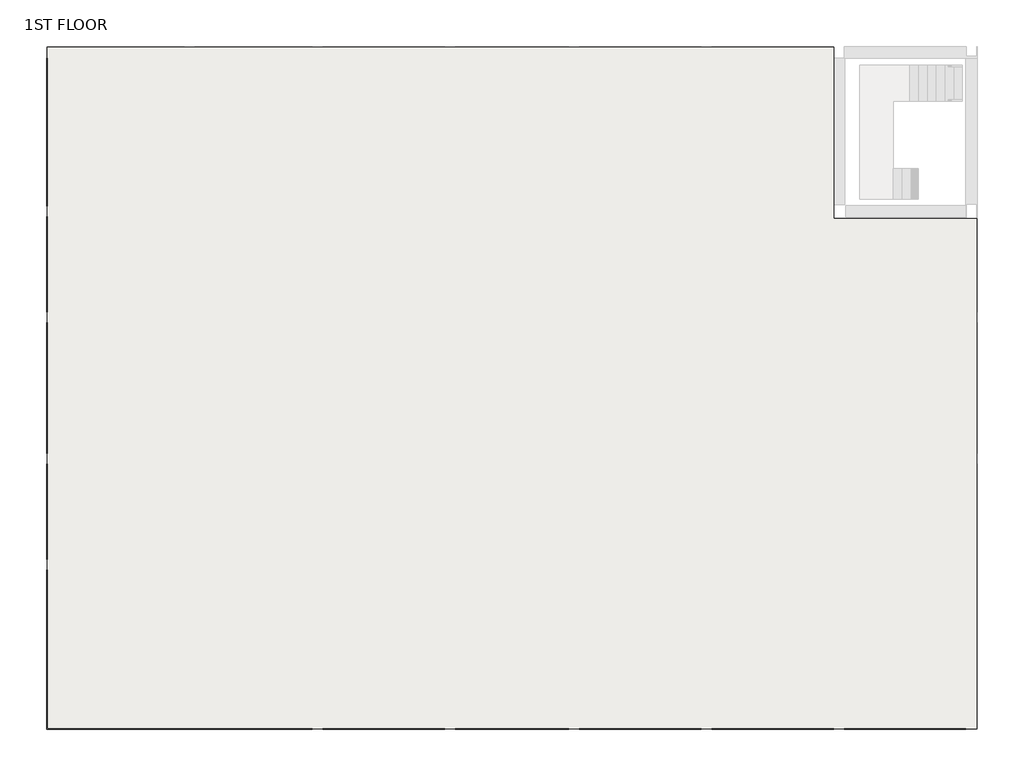
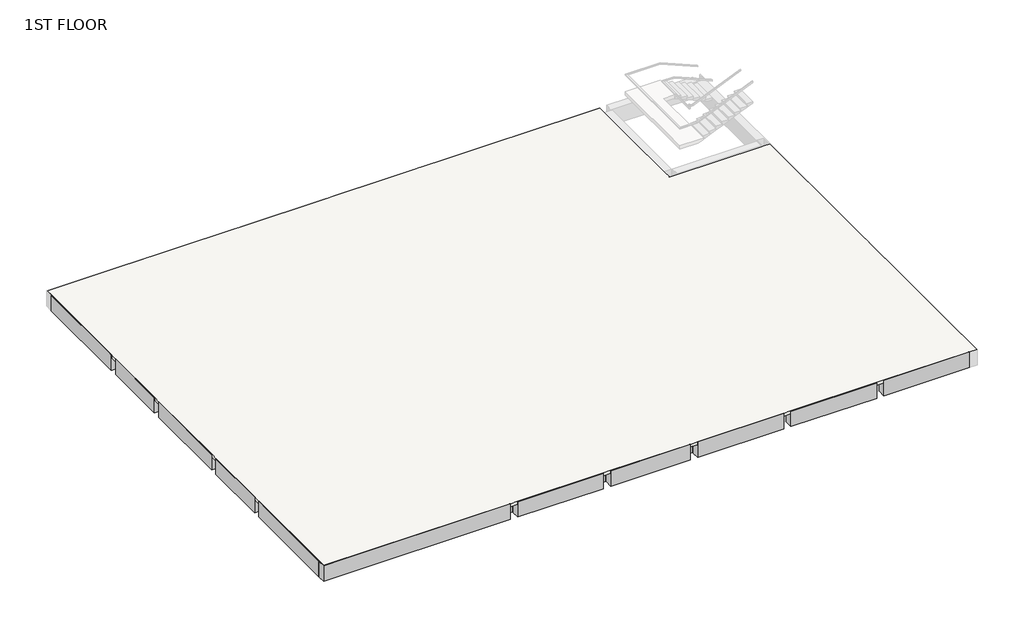
# One storey, part 1 of 2: 9 beams, 1 slab.
"""IFC4 building model written with IfcOpenShell, lengths in millimetres."""

from ifc_helpers import new_model, si_unit, frame, origin, place, context, project, spatial, polyline, outline, extrude, faceted_brep, element, save

model = new_model("IFC4")

# Units and contexts
model_context = context("Model", 3, world=origin())
ifc_project = project(units=[si_unit("LENGTHUNIT", "METRE", prefix="MILLI")], contexts=[model_context])

# Site, building, storey
site = spatial("IfcSite", under=ifc_project)
building = spatial("IfcBuilding", under=site)
storey = spatial("IfcBuildingStorey", under=building, Name="1ST FLOOR", Elevation=4572.0)

# Beams
placement = place(None, origin())
element("IfcBeam", 1, ObjectType="M_Concrete-Rectangular Beam : 400 x 800mm", at=placement, inside=storey, context=model_context, shape_type="Brep", body=[
    faceted_brep([(-25701.5491019, -6047.8309165, 4572.0), (-25701.5491019, -6447.8309165, 4572.0), (-16535.3491019, -6447.8309165, 4572.0), (-16535.3491019, -6425.6309165, 4572.0), (-25679.3491019, -6425.6309165, 4572.0), (-25679.3491019, -6047.8309165, 4572.0), (-25701.5491019, -6047.8309165, 3772.0), (-25679.3491019, -6047.8309165, 4419.6), (-25301.5491019, -6047.8309165, 4419.6), (-20977.1491019, -6047.8309165, 4419.6), (-20577.1491019, -6047.8309165, 4419.6), (-16557.5491019, -6047.8309165, 4419.6), (-16535.3491019, -6047.8309165, 4419.6), (-16535.3491019, -6047.8309165, 3772.0), (-16557.5491019, -6047.8309165, 3772.0), (-20577.1491019, -6047.8309165, 3772.0), (-20977.1491019, -6047.8309165, 3772.0), (-25301.5491019, -6047.8309165, 3772.0), (-25701.5491019, -6447.8309165, 3772.0), (-16535.3491019, -6447.8309165, 3772.0), (-25323.7491019, -6425.6309165, 3772.0), (-25323.7491019, -6070.0309165, 3772.0), (-25679.3491019, -6070.0309165, 3772.0), (-25679.3491019, -6425.6309165, 3772.0), (-20599.3491019, -6425.6309165, 3772.0), (-20599.3491019, -6070.0309165, 3772.0), (-20954.9491019, -6070.0309165, 3772.0), (-20954.9491019, -6425.6309165, 3772.0), (-25323.7491019, -6425.6309165, 4419.6), (-25323.7491019, -6070.0309165, 4419.6), (-16535.3491019, -6425.6309165, 4419.6), (-20599.3491019, -6425.6309165, 4419.6), (-20954.9491019, -6425.6309165, 4419.6), (-25679.3491019, -6425.6309165, 4419.6), (-25679.3491019, -6070.0309165, 4419.6), (-20599.3491019, -6070.0309165, 4419.6), (-20954.9491019, -6070.0309165, 4419.6)], [[[0, 1, 2, 3, 4, 5]], [[6, 0, 5, 7, 8, 9, 10, 11, 12, 13, 14, 15, 16, 17]], [[18, 6, 17, 16, 15, 14, 13, 19], [20, 21, 22, 23], [24, 25, 26, 27]], [[1, 18, 19, 2]], [[1, 0, 6, 18]], [[21, 20, 28, 29]], [[30, 31, 24, 27, 32, 28, 20, 23, 33, 4, 3]], [[4, 33, 23, 22, 34, 7, 5]], [[22, 21, 29, 34]], [[25, 24, 31, 35]], [[27, 26, 36, 32]], [[26, 25, 35, 36]], [[19, 13, 12, 30, 3, 2]], [[28, 32, 36, 35, 31, 30, 12, 11, 10, 9, 8, 7, 34, 29]]]),
    faceted_brep([(5997.6508981, -6447.8309165, 3772.0), (5997.6508981, -6047.8309165, 3772.0), (5997.6508981, -6047.8309165, 4419.6), (5997.6508981, -6425.6309165, 4419.6), (5997.6508981, -6425.6309165, 4572.0), (5997.6508981, -6447.8309165, 4572.0), (1803.4508981, -6047.8309165, 3772.0), (1803.4508981, -6447.8309165, 3772.0), (1803.4508981, -6447.8309165, 4572.0), (1803.4508981, -6425.6309165, 4572.0), (1803.4508981, -6425.6309165, 4419.6), (1803.4508981, -6047.8309165, 4419.6), (1825.6508981, -6047.8309165, 3772.0), (1825.6508981, -6047.8309165, 4419.6)], [[[0, 1, 2, 3, 4, 5]], [[6, 7, 8, 9, 10, 11]], [[8, 5, 4, 9]], [[1, 12, 6, 11, 13, 2]], [[1, 0, 7, 6, 12]], [[0, 5, 8, 7]], [[10, 3, 2, 13, 11]], [[3, 10, 9, 4]]]),
    faceted_brep([(-16179.7491019, -6047.8309165, 3772.0), (-16179.7491019, -6447.8309165, 3772.0), (-16179.7491019, -6447.8309165, 4572.0), (-16179.7491019, -6425.6309165, 4572.0), (-16179.7491019, -6425.6309165, 4419.6), (-16179.7491019, -6047.8309165, 4419.6), (-11963.3491019, -6447.8309165, 4572.0), (-11963.3491019, -6425.6309165, 4572.0), (-11963.3491019, -6047.8309165, 3772.0), (-11985.5491019, -6047.8309165, 3772.0), (-16157.5491019, -6047.8309165, 3772.0), (-16157.5491019, -6047.8309165, 4419.6), (-11985.5491019, -6047.8309165, 4419.6), (-11963.3491019, -6047.8309165, 4419.6), (-11963.3491019, -6447.8309165, 3772.0), (-11963.3491019, -6425.6309165, 4419.6)], [[[0, 1, 2, 3, 4, 5]], [[2, 6, 7, 3]], [[8, 9, 10, 0, 5, 11, 12, 13]], [[1, 0, 10, 9, 8, 14]], [[2, 1, 14, 6]], [[14, 8, 13, 15, 7, 6]], [[15, 4, 3, 7]], [[4, 15, 13, 12, 11, 5]]]),
    faceted_brep([(-11607.7491019, -6047.8309165, 3772.0), (-11607.7491019, -6447.8309165, 3772.0), (-11607.7491019, -6447.8309165, 4572.0), (-11607.7491019, -6425.6309165, 4572.0), (-11607.7491019, -6425.6309165, 4419.6), (-11607.7491019, -6047.8309165, 4419.6), (-7696.1491019, -6447.8309165, 4572.0), (-7696.1491019, -6425.6309165, 4572.0), (-7696.1491019, -6047.8309165, 3772.0), (-7718.3491019, -6047.8309165, 3772.0), (-11585.5491019, -6047.8309165, 3772.0), (-11585.5491019, -6047.8309165, 4419.6), (-7718.3491019, -6047.8309165, 4419.6), (-7696.1491019, -6047.8309165, 4419.6), (-7696.1491019, -6447.8309165, 3772.0), (-7696.1491019, -6425.6309165, 4419.6)], [[[0, 1, 2, 3, 4, 5]], [[2, 6, 7, 3]], [[8, 9, 10, 0, 5, 11, 12, 13]], [[1, 0, 10, 9, 8, 14]], [[2, 1, 14, 6]], [[14, 8, 13, 15, 7, 6]], [[15, 4, 3, 7]], [[4, 15, 13, 12, 11, 5]]]),
    faceted_brep([(-7340.5491019, -6047.8309165, 3772.0), (-7340.5491019, -6447.8309165, 3772.0), (-7340.5491019, -6447.8309165, 4572.0), (-7340.5491019, -6425.6309165, 4572.0), (-7340.5491019, -6425.6309165, 4419.6), (-7340.5491019, -6047.8309165, 4419.6), (-3124.1491019, -6447.8309165, 4572.0), (-3124.1491019, -6425.6309165, 4572.0), (-3124.1491019, -6047.8309165, 3772.0), (-3146.3491019, -6047.8309165, 3772.0), (-7318.3491019, -6047.8309165, 3772.0), (-7318.3491019, -6047.8309165, 4419.6), (-3146.3491019, -6047.8309165, 4419.6), (-3124.1491019, -6047.8309165, 4419.6), (-3124.1491019, -6447.8309165, 3772.0), (-3124.1491019, -6425.6309165, 4419.6)], [[[0, 1, 2, 3, 4, 5]], [[2, 6, 7, 3]], [[8, 9, 10, 0, 5, 11, 12, 13]], [[1, 0, 10, 9, 8, 14]], [[2, 1, 14, 6]], [[14, 8, 13, 15, 7, 6]], [[15, 4, 3, 7]], [[4, 15, 13, 12, 11, 5]]]),
    faceted_brep([(-2768.5491019, -6047.8309165, 3772.0), (-2768.5491019, -6447.8309165, 3772.0), (-2768.5491019, -6447.8309165, 4572.0), (-2768.5491019, -6425.6309165, 4572.0), (-2768.5491019, -6425.6309165, 4419.6), (-2768.5491019, -6047.8309165, 4419.6), (1447.8508981, -6447.8309165, 4572.0), (1447.8508981, -6425.6309165, 4572.0), (1447.8508981, -6047.8309165, 3772.0), (1425.6508981, -6047.8309165, 3772.0), (-2746.3491019, -6047.8309165, 3772.0), (-2746.3491019, -6047.8309165, 4419.6), (1425.6508981, -6047.8309165, 4419.6), (1447.8508981, -6047.8309165, 4419.6), (1447.8508981, -6447.8309165, 3772.0), (1447.8508981, -6425.6309165, 4419.6)], [[[0, 1, 2, 3, 4, 5]], [[2, 6, 7, 3]], [[8, 9, 10, 0, 5, 11, 12, 13]], [[1, 0, 10, 9, 8, 14]], [[2, 1, 14, 6]], [[14, 8, 13, 15, 7, 6]], [[15, 4, 3, 7]], [[4, 15, 13, 12, 11, 5]]]),
])
element("IfcBeam", 2, ObjectType="M_Concrete-Rectangular Beam : 400 x 800mm", at=placement, inside=storey, context=model_context, shape_type="Brep", body=[
    faceted_brep([(-25701.5491019, -939.2309165, 4572.0), (-25701.5491019, -6047.8309165, 4572.0), (-25679.3491019, -6047.8309165, 4572.0), (-25679.3491019, -939.2309165, 4572.0), (-25301.5491019, -6047.8309165, 3772.0), (-25301.5491019, -961.4309165, 3772.0), (-25301.5491019, -939.2309165, 3772.0), (-25301.5491019, -939.2309165, 4419.6), (-25301.5491019, -961.4309165, 4419.6), (-25301.5491019, -6047.8309165, 4419.6), (-25701.5491019, -6047.8309165, 3772.0), (-25701.5491019, -939.2309165, 3772.0), (-25679.3491019, -6047.8309165, 4419.6), (-25679.3491019, -939.2309165, 4419.6)], [[[0, 1, 2, 3]], [[4, 5, 6, 7, 8, 9]], [[4, 10, 11, 6, 5]], [[10, 1, 0, 11]], [[10, 4, 9, 12, 2, 1]], [[6, 11, 0, 3, 13, 7]], [[12, 13, 3, 2]], [[13, 12, 9, 8, 7]]]),
    faceted_brep([(-25301.5491019, 16716.9690835, 3772.0), (-25701.5491019, 16716.9690835, 3772.0), (-25701.5491019, 16716.9690835, 4572.0), (-25679.3491019, 16716.9690835, 4572.0), (-25679.3491019, 16716.9690835, 4419.6), (-25301.5491019, 16716.9690835, 4419.6), (-25701.5491019, 11608.3690835, 4572.0), (-25679.3491019, 11608.3690835, 4572.0), (-25301.5491019, 11608.3690835, 3772.0), (-25301.5491019, 11630.5690835, 3772.0), (-25301.5491019, 11630.5690835, 4419.6), (-25301.5491019, 11608.3690835, 4419.6), (-25701.5491019, 11608.3690835, 3772.0), (-25679.3491019, 11608.3690835, 4419.6)], [[[0, 1, 2, 3, 4, 5]], [[2, 6, 7, 3]], [[8, 9, 0, 5, 10, 11]], [[1, 0, 9, 8, 12]], [[2, 1, 12, 6]], [[12, 8, 11, 13, 7, 6]], [[4, 13, 11, 10, 5]], [[13, 4, 3, 7]]]),
    faceted_brep([(-25701.5491019, 7950.7690835, 3772.0), (-25301.5491019, 7950.7690835, 3772.0), (-25301.5491019, 7950.7690835, 4419.6), (-25679.3491019, 7950.7690835, 4419.6), (-25679.3491019, 7950.7690835, 4572.0), (-25701.5491019, 7950.7690835, 4572.0), (-25301.5491019, 11252.7690835, 3772.0), (-25701.5491019, 11252.7690835, 3772.0), (-25701.5491019, 11252.7690835, 4572.0), (-25679.3491019, 11252.7690835, 4572.0), (-25679.3491019, 11252.7690835, 4419.6), (-25301.5491019, 11252.7690835, 4419.6), (-25301.5491019, 7972.9690835, 4419.6), (-25301.5491019, 11230.5690835, 4419.6), (-25301.5491019, 7972.9690835, 3772.0), (-25301.5491019, 11230.5690835, 3772.0)], [[[0, 1, 2, 3, 4, 5]], [[6, 7, 8, 9, 10, 11]], [[10, 3, 2, 12, 13, 11]], [[3, 10, 9, 4]], [[8, 5, 4, 9]], [[1, 14, 15, 6, 11, 13, 12, 2]], [[1, 0, 7, 6, 15, 14]], [[0, 5, 8, 7]]]),
    faceted_brep([(-25301.5491019, 7595.1690835, 3772.0), (-25701.5491019, 7595.1690835, 3772.0), (-25701.5491019, 7595.1690835, 4572.0), (-25679.3491019, 7595.1690835, 4572.0), (-25679.3491019, 7595.1690835, 4419.6), (-25301.5491019, 7595.1690835, 4419.6), (-25701.5491019, 3073.9690835, 3772.0), (-25301.5491019, 3073.9690835, 3772.0), (-25301.5491019, 3073.9690835, 4419.6), (-25679.3491019, 3073.9690835, 4419.6), (-25679.3491019, 3073.9690835, 4572.0), (-25701.5491019, 3073.9690835, 4572.0), (-25301.5491019, 3096.1690835, 4419.6), (-25301.5491019, 7572.9690835, 4419.6), (-25301.5491019, 3096.1690835, 3772.0), (-25301.5491019, 7572.9690835, 3772.0)], [[[0, 1, 2, 3, 4, 5]], [[6, 7, 8, 9, 10, 11]], [[4, 9, 8, 12, 13, 5]], [[9, 4, 3, 10]], [[2, 11, 10, 3]], [[7, 14, 15, 0, 5, 13, 12, 8]], [[1, 0, 15, 14, 7, 6]], [[2, 1, 6, 11]]]),
    faceted_brep([(-25301.5491019, 2718.3690835, 3772.0), (-25701.5491019, 2718.3690835, 3772.0), (-25701.5491019, 2718.3690835, 4572.0), (-25679.3491019, 2718.3690835, 4572.0), (-25679.3491019, 2718.3690835, 4419.6), (-25301.5491019, 2718.3690835, 4419.6), (-25701.5491019, -583.6309165, 3772.0), (-25301.5491019, -583.6309165, 3772.0), (-25301.5491019, -583.6309165, 4419.6), (-25679.3491019, -583.6309165, 4419.6), (-25679.3491019, -583.6309165, 4572.0), (-25701.5491019, -583.6309165, 4572.0), (-25301.5491019, -561.4309165, 4419.6), (-25301.5491019, 2696.1690835, 4419.6), (-25301.5491019, -561.4309165, 3772.0), (-25301.5491019, 2696.1690835, 3772.0)], [[[0, 1, 2, 3, 4, 5]], [[6, 7, 8, 9, 10, 11]], [[4, 9, 8, 12, 13, 5]], [[9, 4, 3, 10]], [[2, 11, 10, 3]], [[7, 14, 15, 0, 5, 13, 12, 8]], [[0, 15, 14, 7, 6, 1]], [[11, 2, 1, 6]]]),
])
element("IfcBeam", 3, ObjectType="M_Concrete-Rectangular Beam : 400 x 800mm", at=placement, inside=storey, context=model_context, shape_type="SweptSolid", body=[
    extrude(outline(polyline([(-20577.1491019, -6047.8309165), (-20977.1491019, -6047.8309165), (-20977.1491019, -990.0309165), (-20577.1491019, -990.0309165), (-20577.1491019, -6047.8309165)])), frame((0.0, 0.0, 3772.0), z_axis=(0.0, 0.0, 1.0), x_axis=(1.0, 0.0, 0.0)), (0.0, 0.0, 1.0), 647.6),
    extrude(outline(polyline([(-20599.3491019, 16716.9690835), (-20577.1491019, 16716.9690835), (-20577.1491019, 11659.1690835), (-20977.1491019, 11659.1690835), (-20977.1491019, 16716.9690835), (-20954.9491019, 16716.9690835), (-20954.9491019, 16662.9690835), (-20599.3491019, 16662.9690835), (-20599.3491019, 16716.9690835)])), frame((0.0, 0.0, 3772.0), z_axis=(0.0, 0.0, 1.0), x_axis=(1.0, 0.0, 0.0)), (0.0, 0.0, 1.0), 647.6),
    extrude(outline(polyline([(-20977.1491019, 11201.9690835), (-20577.1491019, 11201.9690835), (-20577.1491019, 8001.5690835), (-20977.1491019, 8001.5690835), (-20977.1491019, 11201.9690835)])), frame((0.0, 0.0, 3772.0), z_axis=(0.0, 0.0, 1.0), x_axis=(1.0, 0.0, 0.0)), (0.0, 0.0, 1.0), 647.6),
    extrude(outline(polyline([(-20977.1491019, 7544.3690835), (-20577.1491019, 7544.3690835), (-20577.1491019, 3124.7690835), (-20977.1491019, 3124.7690835), (-20977.1491019, 7544.3690835)])), frame((0.0, 0.0, 3772.0), z_axis=(0.0, 0.0, 1.0), x_axis=(1.0, 0.0, 0.0)), (0.0, 0.0, 1.0), 647.6),
    extrude(outline(polyline([(-20977.1491019, 2667.5690835), (-20577.1491019, 2667.5690835), (-20577.1491019, -532.8309165), (-20977.1491019, -532.8309165), (-20977.1491019, 2667.5690835)])), frame((0.0, 0.0, 3772.0), z_axis=(0.0, 0.0, 1.0), x_axis=(1.0, 0.0, 0.0)), (0.0, 0.0, 1.0), 647.6),
])
element("IfcBeam", 4, ObjectType="M_Concrete-Rectangular Beam : 400 x 800mm", at=placement, inside=storey, context=model_context, shape_type="SweptSolid", body=[
    extrude(outline(polyline([(-16157.5491019, -6047.8309165), (-16179.7491019, -6047.8309165), (-16179.7491019, -6019.2309165), (-16535.3491019, -6019.2309165), (-16535.3491019, -6047.8309165), (-16557.5491019, -6047.8309165), (-16557.5491019, -990.0309165), (-16157.5491019, -990.0309165), (-16157.5491019, -6047.8309165)])), frame((0.0, 0.0, 3772.0), z_axis=(0.0, 0.0, 1.0), x_axis=(1.0, 0.0, 0.0)), (0.0, 0.0, 1.0), 647.6),
    extrude(outline(polyline([(-16179.7491019, 16716.9690835), (-16157.5491019, 16716.9690835), (-16157.5491019, 11659.1690835), (-16557.5491019, 11659.1690835), (-16557.5491019, 16716.9690835), (-16535.3491019, 16716.9690835), (-16535.3491019, 16688.3690835), (-16179.7491019, 16688.3690835), (-16179.7491019, 16716.9690835)])), frame((0.0, 0.0, 3772.0), z_axis=(0.0, 0.0, 1.0), x_axis=(1.0, 0.0, 0.0)), (0.0, 0.0, 1.0), 647.6),
    extrude(outline(polyline([(-16557.5491019, 11201.9690835), (-16157.5491019, 11201.9690835), (-16157.5491019, 8001.5690835), (-16557.5491019, 8001.5690835), (-16557.5491019, 11201.9690835)])), frame((0.0, 0.0, 3772.0), z_axis=(0.0, 0.0, 1.0), x_axis=(1.0, 0.0, 0.0)), (0.0, 0.0, 1.0), 647.6),
    extrude(outline(polyline([(-16557.5491019, 7544.3690835), (-16157.5491019, 7544.3690835), (-16157.5491019, 3124.7690835), (-16557.5491019, 3124.7690835), (-16557.5491019, 7544.3690835)])), frame((0.0, 0.0, 3772.0), z_axis=(0.0, 0.0, 1.0), x_axis=(1.0, 0.0, 0.0)), (0.0, 0.0, 1.0), 647.6),
    extrude(outline(polyline([(-16557.5491019, 2667.5690835), (-16157.5491019, 2667.5690835), (-16157.5491019, -532.8309165), (-16557.5491019, -532.8309165), (-16557.5491019, 2667.5690835)])), frame((0.0, 0.0, 3772.0), z_axis=(0.0, 0.0, 1.0), x_axis=(1.0, 0.0, 0.0)), (0.0, 0.0, 1.0), 647.6),
])
element("IfcBeam", 5, ObjectType="M_Concrete-Rectangular Beam : 400 x 800mm", at=placement, inside=storey, context=model_context, shape_type="SweptSolid", body=[
    extrude(outline(polyline([(-11585.5491019, -6047.8309165), (-11607.7491019, -6047.8309165), (-11607.7491019, -6019.2309165), (-11963.3491019, -6019.2309165), (-11963.3491019, -6047.8309165), (-11985.5491019, -6047.8309165), (-11985.5491019, -990.0309165), (-11585.5491019, -990.0309165), (-11585.5491019, -6047.8309165)])), frame((0.0, 0.0, 3772.0), z_axis=(0.0, 0.0, 1.0), x_axis=(1.0, 0.0, 0.0)), (0.0, 0.0, 1.0), 647.6),
    extrude(outline(polyline([(-11607.7491019, 16716.9690835), (-11585.5491019, 16716.9690835), (-11585.5491019, 11659.1690835), (-11985.5491019, 11659.1690835), (-11985.5491019, 16716.9690835), (-11963.3491019, 16716.9690835), (-11963.3491019, 16688.3690835), (-11607.7491019, 16688.3690835), (-11607.7491019, 16716.9690835)])), frame((0.0, 0.0, 3772.0), z_axis=(0.0, 0.0, 1.0), x_axis=(1.0, 0.0, 0.0)), (0.0, 0.0, 1.0), 647.6),
    extrude(outline(polyline([(-11985.5491019, 11201.9690835), (-11585.5491019, 11201.9690835), (-11585.5491019, 8001.5690835), (-11985.5491019, 8001.5690835), (-11985.5491019, 11201.9690835)])), frame((0.0, 0.0, 3772.0), z_axis=(0.0, 0.0, 1.0), x_axis=(1.0, 0.0, 0.0)), (0.0, 0.0, 1.0), 647.6),
    extrude(outline(polyline([(-11985.5491019, 7544.3690835), (-11585.5491019, 7544.3690835), (-11585.5491019, 3124.7690835), (-11985.5491019, 3124.7690835), (-11985.5491019, 7544.3690835)])), frame((0.0, 0.0, 3772.0), z_axis=(0.0, 0.0, 1.0), x_axis=(1.0, 0.0, 0.0)), (0.0, 0.0, 1.0), 647.6),
    extrude(outline(polyline([(-11585.5491019, -532.8309165), (-11985.5491019, -532.8309165), (-11985.5491019, 2667.5690835), (-11585.5491019, 2667.5690835), (-11585.5491019, -532.8309165)])), frame((0.0, 0.0, 3772.0), z_axis=(0.0, 0.0, 1.0), x_axis=(1.0, 0.0, 0.0)), (0.0, 0.0, 1.0), 647.6),
])
element("IfcBeam", 6, ObjectType="M_Concrete-Rectangular Beam : 400 x 800mm", at=placement, inside=storey, context=model_context, shape_type="SweptSolid", body=[
    extrude(outline(polyline([(-7318.3491019, -6047.8309165), (-7340.5491019, -6047.8309165), (-7340.5491019, -6019.2309165), (-7696.1491019, -6019.2309165), (-7696.1491019, -6047.8309165), (-7718.3491019, -6047.8309165), (-7718.3491019, -990.0309165), (-7318.3491019, -990.0309165), (-7318.3491019, -6047.8309165)])), frame((0.0, 0.0, 3772.0), z_axis=(0.0, 0.0, 1.0), x_axis=(1.0, 0.0, 0.0)), (0.0, 0.0, 1.0), 647.6),
    extrude(outline(polyline([(-7340.5491019, 16716.9690835), (-7318.3491019, 16716.9690835), (-7318.3491019, 11659.1690835), (-7718.3491019, 11659.1690835), (-7718.3491019, 16716.9690835), (-7696.1491019, 16716.9690835), (-7696.1491019, 16688.3690835), (-7340.5491019, 16688.3690835), (-7340.5491019, 16716.9690835)])), frame((0.0, 0.0, 3772.0), z_axis=(0.0, 0.0, 1.0), x_axis=(1.0, 0.0, 0.0)), (0.0, 0.0, 1.0), 647.6),
    extrude(outline(polyline([(-7718.3491019, 7544.3690835), (-7318.3491019, 7544.3690835), (-7318.3491019, 3124.7690835), (-7718.3491019, 3124.7690835), (-7718.3491019, 7544.3690835)])), frame((0.0, 0.0, 3772.0), z_axis=(0.0, 0.0, 1.0), x_axis=(1.0, 0.0, 0.0)), (0.0, 0.0, 1.0), 647.6),
    extrude(outline(polyline([(-7318.3491019, 8001.5690835), (-7718.3491019, 8001.5690835), (-7718.3491019, 11201.9690835), (-7318.3491019, 11201.9690835), (-7318.3491019, 8001.5690835)])), frame((0.0, 0.0, 3772.0), z_axis=(0.0, 0.0, 1.0), x_axis=(1.0, 0.0, 0.0)), (0.0, 0.0, 1.0), 647.6),
    extrude(outline(polyline([(-7318.3491019, -532.8309165), (-7718.3491019, -532.8309165), (-7718.3491019, 2667.5690835), (-7318.3491019, 2667.5690835), (-7318.3491019, -532.8309165)])), frame((0.0, 0.0, 3772.0), z_axis=(0.0, 0.0, 1.0), x_axis=(1.0, 0.0, 0.0)), (0.0, 0.0, 1.0), 647.6),
])
element("IfcBeam", 7, ObjectType="M_Concrete-Rectangular Beam : 400 x 800mm", at=placement, inside=storey, context=model_context, shape_type="SweptSolid", body=[
    extrude(outline(polyline([(-25301.5491019, 3073.9690835), (-25301.5491019, 3096.1690835), (-21005.7491019, 3096.1690835), (-21005.7491019, 2696.1690835), (-25301.5491019, 2696.1690835), (-25301.5491019, 2718.3690835), (-25272.9491019, 2718.3690835), (-25272.9491019, 3073.9690835), (-25301.5491019, 3073.9690835)])), frame((0.0, 0.0, 3772.0), z_axis=(0.0, 0.0, 1.0), x_axis=(1.0, 0.0, 0.0)), (0.0, 0.0, 1.0), 647.6),
    extrude(outline(polyline([(5997.6508981, 3096.1690835), (5997.6508981, 3073.9690835), (5969.0508981, 3073.9690835), (5969.0508981, 2718.3690835), (5997.6508981, 2718.3690835), (5997.6508981, 2696.1690835), (1854.2508981, 2696.1690835), (1854.2508981, 3096.1690835), (5997.6508981, 3096.1690835)])), frame((0.0, 0.0, 3772.0), z_axis=(0.0, 0.0, 1.0), x_axis=(1.0, 0.0, 0.0)), (0.0, 0.0, 1.0), 647.6),
    extrude(outline(polyline([(-20548.5491019, 2696.1690835), (-20548.5491019, 3096.1690835), (-16586.1491019, 3096.1690835), (-16586.1491019, 2696.1690835), (-20548.5491019, 2696.1690835)])), frame((0.0, 0.0, 3772.0), z_axis=(0.0, 0.0, 1.0), x_axis=(1.0, 0.0, 0.0)), (0.0, 0.0, 1.0), 647.6),
    extrude(outline(polyline([(-16128.9491019, 2696.1690835), (-16128.9491019, 3096.1690835), (-12014.1491019, 3096.1690835), (-12014.1491019, 2696.1690835), (-16128.9491019, 2696.1690835)])), frame((0.0, 0.0, 3772.0), z_axis=(0.0, 0.0, 1.0), x_axis=(1.0, 0.0, 0.0)), (0.0, 0.0, 1.0), 647.6),
    extrude(outline(polyline([(1397.0508981, 3096.1690835), (1397.0508981, 2696.1690835), (-2717.7491019, 2696.1690835), (-2717.7491019, 3096.1690835), (1397.0508981, 3096.1690835)])), frame((0.0, 0.0, 3772.0), z_axis=(0.0, 0.0, 1.0), x_axis=(1.0, 0.0, 0.0)), (0.0, 0.0, 1.0), 647.6),
    extrude(outline(polyline([(-3174.9491019, 3096.1690835), (-3174.9491019, 2696.1690835), (-7289.7491019, 2696.1690835), (-7289.7491019, 3096.1690835), (-3174.9491019, 3096.1690835)])), frame((0.0, 0.0, 3772.0), z_axis=(0.0, 0.0, 1.0), x_axis=(1.0, 0.0, 0.0)), (0.0, 0.0, 1.0), 647.6),
    extrude(outline(polyline([(-7746.9491019, 3096.1690835), (-7746.9491019, 2696.1690835), (-11556.9491019, 2696.1690835), (-11556.9491019, 3096.1690835), (-7746.9491019, 3096.1690835)])), frame((0.0, 0.0, 3772.0), z_axis=(0.0, 0.0, 1.0), x_axis=(1.0, 0.0, 0.0)), (0.0, 0.0, 1.0), 647.6),
])
element("IfcBeam", 8, ObjectType="M_Concrete-Rectangular Beam : 400 x 800mm", at=placement, inside=storey, context=model_context, shape_type="SweptSolid", body=[
    extrude(outline(polyline([(-25301.5491019, -583.6309165), (-25301.5491019, -561.4309165), (-21005.7491019, -561.4309165), (-21005.7491019, -961.4309165), (-25301.5491019, -961.4309165), (-25301.5491019, -939.2309165), (-25247.5491019, -939.2309165), (-25247.5491019, -583.6309165), (-25301.5491019, -583.6309165)])), frame((0.0, 0.0, 3772.0), z_axis=(0.0, 0.0, 1.0), x_axis=(1.0, 0.0, 0.0)), (0.0, 0.0, 1.0), 647.6),
    extrude(outline(polyline([(5997.6508981, -561.4309165), (5997.6508981, -961.4309165), (1854.2508981, -961.4309165), (1854.2508981, -561.4309165), (5997.6508981, -561.4309165)])), frame((0.0, 0.0, 3772.0), z_axis=(0.0, 0.0, 1.0), x_axis=(1.0, 0.0, 0.0)), (0.0, 0.0, 1.0), 647.6),
    extrude(outline(polyline([(-20548.5491019, -961.4309165), (-20548.5491019, -561.4309165), (-16586.1491019, -561.4309165), (-16586.1491019, -961.4309165), (-20548.5491019, -961.4309165)])), frame((0.0, 0.0, 3772.0), z_axis=(0.0, 0.0, 1.0), x_axis=(1.0, 0.0, 0.0)), (0.0, 0.0, 1.0), 647.6),
    extrude(outline(polyline([(-16128.9491019, -961.4309165), (-16128.9491019, -561.4309165), (-12014.1491019, -561.4309165), (-12014.1491019, -961.4309165), (-16128.9491019, -961.4309165)])), frame((0.0, 0.0, 3772.0), z_axis=(0.0, 0.0, 1.0), x_axis=(1.0, 0.0, 0.0)), (0.0, 0.0, 1.0), 647.6),
    extrude(outline(polyline([(-11556.9491019, -961.4309165), (-11556.9491019, -561.4309165), (-7746.9491019, -561.4309165), (-7746.9491019, -961.4309165), (-11556.9491019, -961.4309165)])), frame((0.0, 0.0, 3772.0), z_axis=(0.0, 0.0, 1.0), x_axis=(1.0, 0.0, 0.0)), (0.0, 0.0, 1.0), 647.6),
    extrude(outline(polyline([(-7289.7491019, -961.4309165), (-7289.7491019, -561.4309165), (-3174.9491019, -561.4309165), (-3174.9491019, -961.4309165), (-7289.7491019, -961.4309165)])), frame((0.0, 0.0, 3772.0), z_axis=(0.0, 0.0, 1.0), x_axis=(1.0, 0.0, 0.0)), (0.0, 0.0, 1.0), 647.6),
    extrude(outline(polyline([(-2717.7491019, -961.4309165), (-2717.7491019, -561.4309165), (1397.0508981, -561.4309165), (1397.0508981, -961.4309165), (-2717.7491019, -961.4309165)])), frame((0.0, 0.0, 3772.0), z_axis=(0.0, 0.0, 1.0), x_axis=(1.0, 0.0, 0.0)), (0.0, 0.0, 1.0), 647.6),
])
element("IfcBeam", 9, ObjectType="M_Concrete-Rectangular Beam : 400 x 800mm", at=placement, inside=storey, context=model_context, shape_type="SweptSolid", body=[
    extrude(outline(polyline([(-25301.5491019, 7950.7690835), (-25301.5491019, 7972.9690835), (-21005.7491019, 7972.9690835), (-21005.7491019, 7572.9690835), (-25301.5491019, 7572.9690835), (-25301.5491019, 7595.1690835), (-25272.9491019, 7595.1690835), (-25272.9491019, 7950.7690835), (-25301.5491019, 7950.7690835)])), frame((0.0, 0.0, 3772.0), z_axis=(0.0, 0.0, 1.0), x_axis=(1.0, 0.0, 0.0)), (0.0, 0.0, 1.0), 647.6),
    extrude(outline(polyline([(5997.6508981, 7972.9690835), (5997.6508981, 7950.7690835), (5969.0508981, 7950.7690835), (5969.0508981, 7595.1690835), (5997.6508981, 7595.1690835), (5997.6508981, 7572.9690835), (1854.2508981, 7572.9690835), (1854.2508981, 7972.9690835), (5997.6508981, 7972.9690835)])), frame((0.0, 0.0, 3772.0), z_axis=(0.0, 0.0, 1.0), x_axis=(1.0, 0.0, 0.0)), (0.0, 0.0, 1.0), 647.6),
    extrude(outline(polyline([(-7289.7491019, 7572.9690835), (-7289.7491019, 7972.9690835), (-3174.9491019, 7972.9690835), (-3174.9491019, 7572.9690835), (-7289.7491019, 7572.9690835)])), frame((0.0, 0.0, 3772.0), z_axis=(0.0, 0.0, 1.0), x_axis=(1.0, 0.0, 0.0)), (0.0, 0.0, 1.0), 647.6),
    extrude(outline(polyline([(-7746.9491019, 7972.9690835), (-7746.9491019, 7572.9690835), (-11556.9491019, 7572.9690835), (-11556.9491019, 7972.9690835), (-7746.9491019, 7972.9690835)])), frame((0.0, 0.0, 3772.0), z_axis=(0.0, 0.0, 1.0), x_axis=(1.0, 0.0, 0.0)), (0.0, 0.0, 1.0), 647.6),
    extrude(outline(polyline([(1397.0508981, 7972.9690835), (1397.0508981, 7572.9690835), (-2717.7491019, 7572.9690835), (-2717.7491019, 7972.9690835), (1397.0508981, 7972.9690835)])), frame((0.0, 0.0, 3772.0), z_axis=(0.0, 0.0, 1.0), x_axis=(1.0, 0.0, 0.0)), (0.0, 0.0, 1.0), 647.6),
    extrude(outline(polyline([(-12014.1491019, 7972.9690835), (-12014.1491019, 7572.9690835), (-16128.9491019, 7572.9690835), (-16128.9491019, 7972.9690835), (-12014.1491019, 7972.9690835)])), frame((0.0, 0.0, 3772.0), z_axis=(0.0, 0.0, 1.0), x_axis=(1.0, 0.0, 0.0)), (0.0, 0.0, 1.0), 647.6),
    extrude(outline(polyline([(-16586.1491019, 7972.9690835), (-16586.1491019, 7572.9690835), (-20548.5491019, 7572.9690835), (-20548.5491019, 7972.9690835), (-16586.1491019, 7972.9690835)])), frame((0.0, 0.0, 3772.0), z_axis=(0.0, 0.0, 1.0), x_axis=(1.0, 0.0, 0.0)), (0.0, 0.0, 1.0), 647.6),
])

# Slab
element("IfcSlab", 10, ObjectType="6\" Foundation Slab", at=placement, inside=storey, context=model_context, shape_type="Brep", body=[
    faceted_brep([(6375.4508981, -6425.6309165, 4419.6), (6019.8508981, -6425.6309165, 4419.6), (5997.6508981, -6425.6309165, 4419.6), (1803.4508981, -6425.6309165, 4419.6), (1447.8508981, -6425.6309165, 4419.6), (-2768.5491019, -6425.6309165, 4419.6), (-3124.1491019, -6425.6309165, 4419.6), (-7340.5491019, -6425.6309165, 4419.6), (-7696.1491019, -6425.6309165, 4419.6), (-11607.7491019, -6425.6309165, 4419.6), (-11963.3491019, -6425.6309165, 4419.6), (-16179.7491019, -6425.6309165, 4419.6), (-16535.3491019, -6425.6309165, 4419.6), (-20599.3491019, -6425.6309165, 4419.6), (-20954.9491019, -6425.6309165, 4419.6), (-25323.7491019, -6425.6309165, 4419.6), (-25679.3491019, -6425.6309165, 4419.6), (-25679.3491019, -6070.0309165, 4419.6), (-25679.3491019, -6047.8309165, 4419.6), (-25679.3491019, -939.2309165, 4419.6), (-25679.3491019, -583.6309165, 4419.6), (-25679.3491019, 2718.3690835, 4419.6), (-25679.3491019, 3073.9690835, 4419.6), (-25679.3491019, 7595.1690835, 4419.6), (-25679.3491019, 7950.7690835, 4419.6), (-25679.3491019, 11252.7690835, 4419.6), (-25679.3491019, 11608.3690835, 4419.6), (-25679.3491019, 16716.9690835, 4419.6), (-25679.3491019, 16739.1690835, 4419.6), (-25679.3491019, 17094.7690835, 4419.6), (-25323.7491019, 17094.7690835, 4419.6), (-20954.9491019, 17094.7690835, 4419.6), (-20599.3491019, 17094.7690835, 4419.6), (-16535.3491019, 17094.7690835, 4419.6), (-16179.7491019, 17094.7690835, 4419.6), (-11963.3491019, 17094.7690835, 4419.6), (-11607.7491019, 17094.7690835, 4419.6), (-7696.1491019, 17094.7690835, 4419.6), (-7340.5491019, 17094.7690835, 4419.6), (-3124.1491019, 17094.7690835, 4419.6), (-2768.5491019, 17094.7690835, 4419.6), (1447.8508981, 17094.7690835, 4419.6), (1447.8508981, 16716.9690835, 4419.6), (1447.8508981, 16713.7690835, 4419.6), (1447.8508981, 11659.1690835, 4419.6), (1447.8508981, 11201.9690835, 4419.6), (1447.8508981, 11176.5690835, 4419.6), (1825.6508981, 11176.5690835, 4419.6), (5997.6508981, 11176.5690835, 4419.6), (6019.8508981, 11176.5690835, 4419.6), (6375.4508981, 11176.5690835, 4419.6), (6375.4508981, 7950.7690835, 4419.6), (6375.4508981, 7595.1690835, 4419.6), (6375.4508981, 3073.9690835, 4419.6), (6375.4508981, 2718.3690835, 4419.6), (6375.4508981, -507.4309165, 4419.6), (6375.4508981, -1015.4309165, 4419.6), (6375.4508981, -6070.0309165, 4419.6), (-25679.3491019, -6425.6309165, 4572.0), (-16535.3491019, -6425.6309165, 4572.0), (-16179.7491019, -6425.6309165, 4572.0), (-11963.3491019, -6425.6309165, 4572.0), (-11607.7491019, -6425.6309165, 4572.0), (-7696.1491019, -6425.6309165, 4572.0), (-7340.5491019, -6425.6309165, 4572.0), (-3124.1491019, -6425.6309165, 4572.0), (-2768.5491019, -6425.6309165, 4572.0), (1447.8508981, -6425.6309165, 4572.0), (1803.4508981, -6425.6309165, 4572.0), (5997.6508981, -6425.6309165, 4572.0), (6375.4508981, -6425.6309165, 4572.0), (6375.4508981, 2718.3690835, 4572.0), (6375.4508981, 3073.9690835, 4572.0), (6375.4508981, 7595.1690835, 4572.0), (6375.4508981, 7950.7690835, 4572.0), (6375.4508981, 11176.5690835, 4572.0), (6019.8508981, 11176.5690835, 4572.0), (5997.6508981, 11176.5690835, 4572.0), (1825.6508981, 11176.5690835, 4572.0), (1447.8508981, 11176.5690835, 4572.0), (1447.8508981, 11201.9690835, 4572.0), (1447.8508981, 11659.1690835, 4572.0), (1447.8508981, 16713.7690835, 4572.0), (1447.8508981, 17094.7690835, 4572.0), (-2768.5491019, 17094.7690835, 4572.0), (-3124.1491019, 17094.7690835, 4572.0), (-7340.5491019, 17094.7690835, 4572.0), (-7696.1491019, 17094.7690835, 4572.0), (-11607.7491019, 17094.7690835, 4572.0), (-11963.3491019, 17094.7690835, 4572.0), (-16179.7491019, 17094.7690835, 4572.0), (-16535.3491019, 17094.7690835, 4572.0), (-20599.3491019, 17094.7690835, 4572.0), (-20954.9491019, 17094.7690835, 4572.0), (-25679.3491019, 17094.7690835, 4572.0), (-25679.3491019, 16716.9690835, 4572.0), (-25679.3491019, 11608.3690835, 4572.0), (-25679.3491019, 11252.7690835, 4572.0), (-25679.3491019, 7950.7690835, 4572.0), (-25679.3491019, 7595.1690835, 4572.0), (-25679.3491019, 3073.9690835, 4572.0), (-25679.3491019, 2718.3690835, 4572.0), (-25679.3491019, -583.6309165, 4572.0), (-25679.3491019, -939.2309165, 4572.0), (-25679.3491019, -6047.8309165, 4572.0)], [[[0, 1, 2, 3, 4, 5, 6, 7, 8, 9, 10, 11, 12, 13, 14, 15, 16, 17, 18, 19, 20, 21, 22, 23, 24, 25, 26, 27, 28, 29, 30, 31, 32, 33, 34, 35, 36, 37, 38, 39, 40, 41, 42, 43, 44, 45, 46, 47, 48, 49, 50, 51, 52, 53, 54, 55, 56, 57]], [[58, 59, 60, 61, 62, 63, 64, 65, 66, 67, 68, 69, 70, 71, 72, 73, 74, 75, 76, 77, 78, 79, 80, 81, 82, 83, 84, 85, 86, 87, 88, 89, 90, 91, 92, 93, 94, 95, 96, 97, 98, 99, 100, 101, 102, 103, 104]], [[70, 0, 57, 56, 55, 54, 53, 52, 51, 50, 75, 74, 73, 72, 71]], [[16, 15, 14, 13, 12, 11, 10, 9, 8, 7, 6, 5, 4, 3, 2, 1, 0, 70, 69, 68, 67, 66, 65, 64, 63, 62, 61, 60, 59, 58]], [[29, 28, 27, 26, 25, 24, 23, 22, 21, 20, 19, 18, 17, 16, 58, 104, 103, 102, 101, 100, 99, 98, 97, 96, 95, 94]], [[29, 94, 93, 92, 91, 90, 89, 88, 87, 86, 85, 84, 83, 41, 40, 39, 38, 37, 36, 35, 34, 33, 32, 31, 30]], [[79, 46, 45, 44, 43, 42, 41, 83, 82, 81, 80]], [[46, 79, 78, 77, 76, 75, 50, 49, 48, 47]]]),
])

save(model, "model.ifc")

# Revit data of these elements
# Type "M_Concrete-Rectangular Beam : 400 x 800mm"
#   Length [instance default] = 5' - 0"
#   b = 1' - 3.74803"
#   h = 2' - 7.49606"
#   Structural Material [instance default] = Concrete, Cast-in-Place gray
#   Assembly Code = ""
# Type "6\" Foundation Slab"
#   Layers, outside or top first: 0' - 6" "Concrete, Cast-in-Place gray" (function 1)
# Elements 1, 2 (IfcBeam, "M_Concrete-Rectangular Beam : 400 x 800mm")
#   Structural Material = Concrete, Cast-in-Place gray
#   Phase Created = New Construction
#   Materials on its faces: "Concrete, Cast-in-Place gray"
# Elements 3, 4, 5, 6, 7, 8, 9 (IfcBeam, "M_Concrete-Rectangular Beam : 400 x 800mm")
#   Comments = ""
#   Structural Material = Concrete, Cast-in-Place gray
#   Phase Created = New Construction
#   Materials on its faces: "Concrete, Cast-in-Place gray"
# Element 10 (IfcSlab, "6\" Foundation Slab")
#   Height Offset From Level = 0' - 0"
#   built-in parameter 1001954 = 1
#   Phase Created = New Construction
#   Materials on its faces: "Concrete, Cast-in-Place gray"
# Materials
#   "Concrete, Cast-in-Place gray": class "Concrete", colour RGB 192 192 192, transparency 0, Description = "Cast-in-place concrete", Cost = 0
